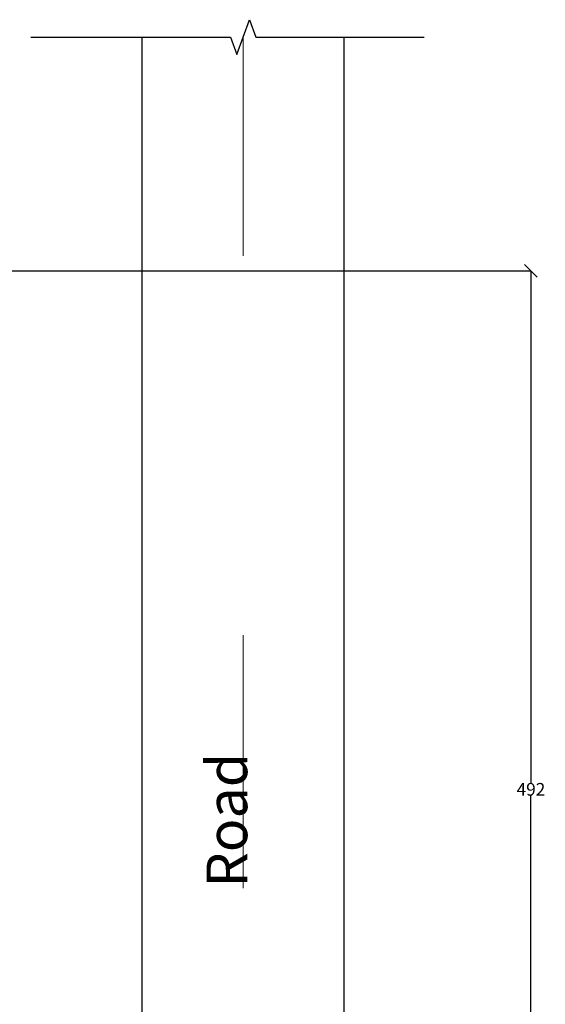
# Model space of a CAD drawing. Units: inches. Extents: x -1198 to -69, y -512 to 437.
# Tile 50 of 50: x -322 to -73, y -85 to 382. Entities that reach past the tile are written whole.
import ezdxf

# ---------------------------------------------------------------- set-up
doc = ezdxf.new("R2010")
doc.units = ezdxf.units.IN
doc.header["$MEASUREMENT"] = 0
doc.linetypes.add('ACAD_ISO03W100', pattern=[30, 12, -18])
for name, color, linetype, lineweight in [('A-ANNO-DIMS', 2, 'Continuous', 18), ('A-ANNO-TEXT', 7, 'Continuous', 25), ('C-ROAD', 7, 'Continuous', 25), ('C-ROAD-CNTR', 7, 'ACAD_ISO03W100', 18)]:
    doc.layers.add(name, color=color, linetype=linetype, lineweight=lineweight)
doc.styles.get("Standard").update_dxf_attribs({"font": 'arial.ttf'})
doc.dimstyles.get("Standard").update_dxf_attribs({"dimtxt": 6, "dimasz": 6, "dimexe": 0.18, "dimexo": 0.0625, "dimgap": 0.09, "dimtad": 0, "dimtih": 1, "dimtoh": 1, "dimdec": 0, "dimzin": 0, "dimdsep": 46, "dimlunit": 4, "dimtxsty": 'Standard', "dimblk": 'OBLIQUE', "dimcen": 0.09, "dimadec": 0, "dimazin": 0, "dimtfac": 1, "dimtdec": 0, "dimtofl": 0, "dimtmove": 0, "dimatfit": 3, "dimfxl": 1, "dimtolj": 1, "dimtzin": 0, "dimarcsym": 0})

# ---------------------------------------------------------------- blocks, each defined once
blk = doc.blocks.new('_Oblique')
at = {"color": 0, "linetype": 'ByBlock', "lineweight": -2}
blk.add_line((-0.5, -0.5), (0.5, 0.5), dxfattribs=at)
blk = doc.blocks.new('*D63')
at = {"layer": 'A-ANNO-DIMS', "color": 0, "lineweight": -2, "ltscale": 10, "transparency": 16777216}
for p, q in [((-370.69, 263.23), (-79.37, 263.23)), ((-79.55, 263.23), (-79.55, 20.38)), ((-79.55, -228.77), (-79.55, 14.07)), ((-370.69, -228.77), (-79.37, -228.77))]:
    blk.add_line(p, q, dxfattribs=at)
at = {"layer": 'DEFPOINTS', "color": 0, "ltscale": 10, "transparency": 16777216}
for p in [(-370.75, 263.23), (-79.55, 263.23), (-370.75, -228.77)]:
    blk.add_point(p, dxfattribs=at)
at = {"layer": 'A-ANNO-DIMS', "color": 0, "lineweight": -2, "ltscale": 10, "transparency": 16777216, "xscale": 6, "yscale": 6, "zscale": 6}
for p, rotation in [((-79.55, 263.23), 90), ((-79.55, -228.77), 270)]:
    blk.add_blockref('_Oblique', p, dxfattribs=dict(at, rotation=rotation))
at = {"layer": 'A-ANNO-DIMS', "color": 0, "ltscale": 10, "transparency": 16777216, "insert": (-79.55, 17.23), "char_height": 6, "attachment_point": 5}
blk.add_mtext('\\A1;492', dxfattribs=at)

msp = doc.modelspace()

# ---------------------------------------------------------------- linework, layer by layer
at = {"layer": 'C-ROAD', "ltscale": 10}
for p, q in [((-264.1167, -329.6039), (-264.1167, 374.1612)), ((-168.1167, -425.6039), (-168.1167, 374.1612))]:
    msp.add_line(p, q, dxfattribs=at)
msp.add_lwpolyline([(-316.8761, 374.1612), (-222.1167, 374.1612), (-219.1167, 365.9188), (-213.1167, 382.4036), (-210.1167, 374.1612), (-130.1507, 374.1612)], dxfattribs=at)
at = {"layer": 'C-ROAD-CNTR', "ltscale": 10}
msp.add_line((-216.1167, -329.6039), (-216.1167, 374.1612), dxfattribs=at)

# ---------------------------------------------------------------- texts
at = {"layer": 'A-ANNO-TEXT', "ltscale": 10, "insert": (-233.5093, -29.3306), "char_height": 19.32196, "attachment_point": 1, "rotation": 90}
msp.add_mtext_dynamic_manual_height_columns('Road', width=186.703358, gutter_width=96.6098, heights=[0], dxfattribs=at)

# ---------------------------------------------------------------- dimensions: what is measured, and where the dimension line sits
at = {"layer": 'A-ANNO-DIMS', "ltscale": 10}
dim = msp.add_linear_dim(base=(-79.5507, 263.2277), p1=(-370.7509, -228.7723), p2=(-370.7509, 263.2277), angle=90, dimstyle='Standard', override={"dimdec": 0, "dimlfac": 1, "dimrnd": 0, "dimzin": 0, "dimdsep": 46, "dimlunit": 2}, dxfattribs=at)
dim.commit()
dim.dimension.update_dxf_attribs({"geometry": '*D63', "text_midpoint": (-79.5507, 17.2277)})

doc.saveas('drawing.dxf')
